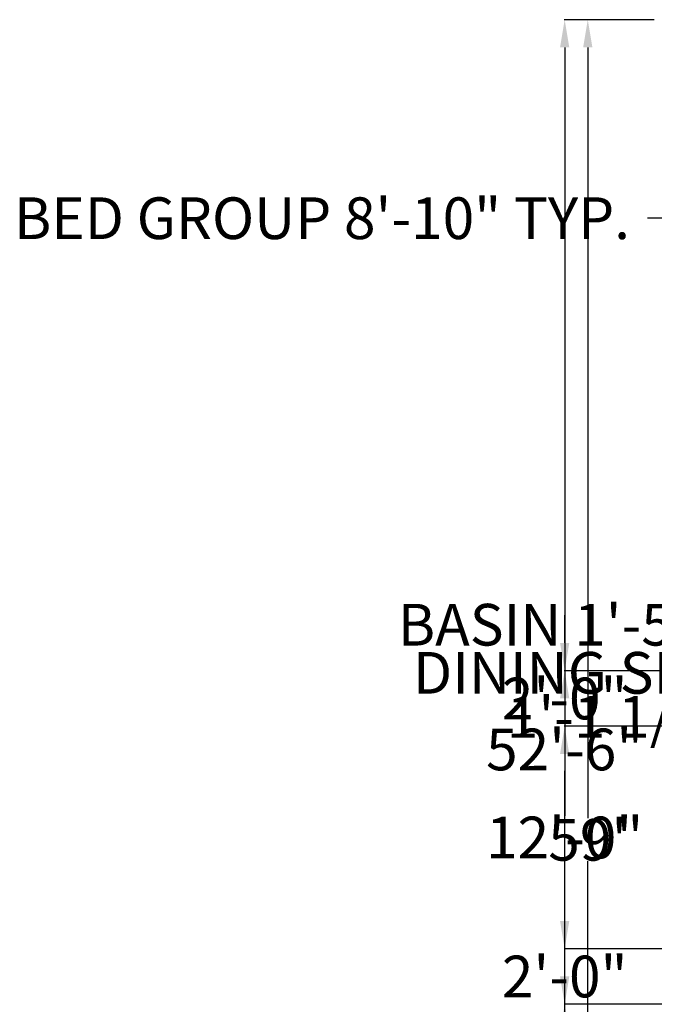
# Model space of a CAD drawing. Units: inches. Extents: x 2796 to 3603, y 978 to 1787.
# Tile 7 of 15: x 2796 to 3070, y 1312 to 1737. Entities that reach past the tile are written whole.
import ezdxf

# ---------------------------------------------------------------- set-up
doc = ezdxf.new("R2010")
doc.units = ezdxf.units.IN
doc.layers.add('A-ANNO-DIMS', color=7, linetype='Continuous', lineweight=18)
doc.styles.get("Standard").update_dxf_attribs({"font": 'arial.ttf'})
doc.dimstyles.get("Standard").update_dxf_attribs({"dimtxt": 18, "dimasz": 12, "dimexe": 0.18, "dimexo": 0.0625, "dimgap": 0.09, "dimtad": 0, "dimtih": 1, "dimtoh": 1, "dimdec": 0, "dimzin": 0, "dimdsep": 46, "dimlunit": 3, "dimtxsty": 'Standard', "dimcen": 0.09, "dimadec": 0, "dimazin": 0, "dimtfac": 1, "dimtdec": 0, "dimtofl": 0, "dimtmove": 0, "dimatfit": 3, "dimfxl": 1, "dimtolj": 1, "dimtzin": 0, "dimarcsym": 0})

# ---------------------------------------------------------------- blocks, each defined once
blk = doc.blocks.new('*D12')
at = {"layer": 'A-ANNO-DIMS', "color": 0, "lineweight": -2, "transparency": 16777216}
for p, q in [((3070.18, 1736.68), (3041.33, 1736.68)), ((3041.51, 1724.68), (3041.51, 1391.96)), ((3041.51, 1040.68), (3041.51, 1373.4)), ((3070.18, 1028.68), (3041.33, 1028.68))]:
    blk.add_line(p, q, dxfattribs=at)
at = {"layer": 'A-ANNO-DIMS', "color": 0, "transparency": 16777216}
for points in [[(3039.51, 1724.68), (3043.51, 1724.68), (3041.51, 1736.68)], [(3039.51, 1040.68), (3043.51, 1040.68), (3041.51, 1028.68)]]:
    blk.add_solid(points, dxfattribs=at)
at = {"layer": 'Defpoints', "color": 0, "transparency": 16777216}
for p in [(3041.51, 1736.68), (3070.25, 1736.68), (3070.25, 1028.68)]:
    blk.add_point(p, dxfattribs=at)
at = {"layer": 'A-ANNO-DIMS', "color": 0, "transparency": 16777216, "insert": (3041.51, 1382.68), "char_height": 18, "attachment_point": 5}
blk.add_mtext("\\A1;59'", dxfattribs=at)
blk = doc.blocks.new('*D22')
at = {"layer": 'A-ANNO-DIMS', "color": 0, "lineweight": -2, "transparency": 16777216}
for p, q in [((3160.28, 1475.52), (3148.28, 1475.52)), ((3172.28, 1473.07), (3172.28, 1475.7)), ((3189.07, 1473.07), (3189.07, 1475.7)), ((3201.07, 1475.52), (3213.07, 1475.52))]:
    blk.add_line(p, q, dxfattribs=at)
at = {"layer": 'A-ANNO-DIMS', "color": 0, "transparency": 16777216}
for points in [[(3160.28, 1477.52), (3160.28, 1473.52), (3172.28, 1475.52)], [(3201.07, 1477.52), (3201.07, 1473.52), (3189.07, 1475.52)]]:
    blk.add_solid(points, dxfattribs=at)
at = {"layer": 'Defpoints', "color": 0, "transparency": 16777216}
for p in [(3172.28, 1475.52), (3172.28, 1473), (3189.07, 1473)]:
    blk.add_point(p, dxfattribs=at)
at = {"layer": 'A-ANNO-DIMS', "color": 0, "transparency": 16777216, "insert": (3052.51, 1475.52), "char_height": 18, "attachment_point": 5}
blk.add_mtext('\\A1;BASIN 1\'-5" TYP.', dxfattribs=at)
blk = doc.blocks.new('*D23')
at = {"layer": 'A-ANNO-DIMS', "color": 0, "lineweight": -2, "transparency": 16777216}
for p, q in [((3169.76, 1485), (3169.76, 1497)), ((3172.22, 1473), (3169.58, 1473)), ((3172.22, 1459.7), (3169.58, 1459.7)), ((3169.76, 1447.7), (3169.76, 1435.7)), ((3169.76, 1435.7), (3157.76, 1435.7))]:
    blk.add_line(p, q, dxfattribs=at)
at = {"layer": 'A-ANNO-DIMS', "color": 0, "transparency": 16777216}
for points in [[(3167.76, 1485), (3171.76, 1485), (3169.76, 1473)], [(3167.76, 1447.7), (3171.76, 1447.7), (3169.76, 1459.7)]]:
    blk.add_solid(points, dxfattribs=at)
at = {"layer": 'Defpoints', "color": 0, "transparency": 16777216}
for p in [(3172.28, 1473), (3169.76, 1459.7), (3172.28, 1459.7)]:
    blk.add_point(p, dxfattribs=at)
at = {"layer": 'A-ANNO-DIMS', "color": 0, "transparency": 16777216, "insert": (3082.69, 1435.7), "char_height": 18, "attachment_point": 5}
blk.add_mtext('\\A1;1\'-1 1/2" TYP.', dxfattribs=at)
blk = doc.blocks.new('*D26')
at = {"layer": 'A-ANNO-DIMS', "color": 0, "lineweight": -2, "transparency": 16777216}
for p, q in [((3079.25, 1650.99), (3067.25, 1650.99)), ((3079.25, 1635.16), (3079.25, 1651.17)), ((3173.2, 1650.99), (3091.25, 1650.99)), ((3185.2, 1635.16), (3185.2, 1651.17))]:
    blk.add_line(p, q, dxfattribs=at)
at = {"layer": 'A-ANNO-DIMS', "color": 0, "transparency": 16777216}
for points in [[(3091.25, 1652.99), (3091.25, 1648.99), (3079.25, 1650.99)], [(3173.2, 1652.99), (3173.2, 1648.99), (3185.2, 1650.99)]]:
    blk.add_solid(points, dxfattribs=at)
at = {"layer": 'Defpoints', "color": 0, "transparency": 16777216}
for p in [(3079.25, 1650.99), (3079.25, 1635.1), (3185.2, 1635.1)]:
    blk.add_point(p, dxfattribs=at)
at = {"layer": 'A-ANNO-DIMS', "color": 0, "transparency": 16777216, "insert": (2926.76, 1650.99), "char_height": 18, "attachment_point": 5}
blk.add_mtext('\\A1;BED GROUP 8\'-10" TYP.', dxfattribs=at)
blk = doc.blocks.new('*D32')
at = {"layer": 'A-ANNO-DIMS', "color": 0, "lineweight": -2, "transparency": 16777216}
for p, q in [((3229.46, 1454.75), (3217.46, 1454.75)), ((3229.46, 1444.07), (3229.46, 1454.93)), ((3289.09, 1454.75), (3241.46, 1454.75)), ((3301.09, 1444.07), (3301.09, 1454.93))]:
    blk.add_line(p, q, dxfattribs=at)
at = {"layer": 'A-ANNO-DIMS', "color": 0, "transparency": 16777216}
for points in [[(3241.46, 1456.75), (3241.46, 1452.75), (3229.46, 1454.75)], [(3289.09, 1456.75), (3289.09, 1452.75), (3301.09, 1454.75)]]:
    blk.add_solid(points, dxfattribs=at)
at = {"layer": 'Defpoints', "color": 0, "transparency": 16777216}
for p in [(3229.46, 1454.75), (3229.46, 1444.01), (3301.09, 1444.01)]:
    blk.add_point(p, dxfattribs=at)
at = {"layer": 'A-ANNO-DIMS', "color": 0, "transparency": 16777216, "insert": (3090.48, 1454.75), "char_height": 18, "attachment_point": 5}
blk.add_mtext('\\A1;DINING SET 5\'-11 1/2"', dxfattribs=at)
blk = doc.blocks.new('*D41')
at = {"layer": 'A-ANNO-DIMS', "color": 0, "lineweight": -2, "transparency": 16777216}
for p, q in [((3079.18, 1455.68), (3031.37, 1455.68)), ((3031.55, 1443.68), (3031.55, 1392.96)), ((3031.55, 1323.68), (3031.55, 1374.4)), ((3079.18, 1311.68), (3031.37, 1311.68))]:
    blk.add_line(p, q, dxfattribs=at)
at = {"layer": 'A-ANNO-DIMS', "color": 0, "transparency": 16777216}
for points in [[(3029.55, 1443.68), (3033.55, 1443.68), (3031.55, 1455.68)], [(3029.55, 1323.68), (3033.55, 1323.68), (3031.55, 1311.68)]]:
    blk.add_solid(points, dxfattribs=at)
at = {"layer": 'Defpoints', "color": 0, "transparency": 16777216}
for p in [(3031.55, 1455.68), (3079.25, 1455.68), (3079.25, 1311.68)]:
    blk.add_point(p, dxfattribs=at)
at = {"layer": 'A-ANNO-DIMS', "color": 0, "transparency": 16777216, "insert": (3031.55, 1383.68), "char_height": 18, "attachment_point": 5}
blk.add_mtext('\\A1;12\'-0"', dxfattribs=at)
blk = doc.blocks.new('*D45')
at = {"layer": 'A-ANNO-DIMS', "color": 0, "lineweight": -2, "transparency": 16777216}
for p, q in [((3070.18, 1736.68), (3031.37, 1736.68)), ((3031.55, 1724.68), (3031.55, 1430.96)), ((3031.55, 1118.68), (3031.55, 1412.4)), ((3070.18, 1106.68), (3031.37, 1106.68))]:
    blk.add_line(p, q, dxfattribs=at)
at = {"layer": 'A-ANNO-DIMS', "color": 0, "transparency": 16777216}
for points in [[(3029.55, 1724.68), (3033.55, 1724.68), (3031.55, 1736.68)], [(3029.55, 1118.68), (3033.55, 1118.68), (3031.55, 1106.68)]]:
    blk.add_solid(points, dxfattribs=at)
at = {"layer": 'Defpoints', "color": 0, "transparency": 16777216}
for p in [(3031.55, 1736.68), (3070.25, 1736.68), (3070.25, 1106.68)]:
    blk.add_point(p, dxfattribs=at)
at = {"layer": 'A-ANNO-DIMS', "color": 0, "transparency": 16777216, "insert": (3031.55, 1421.68), "char_height": 18, "attachment_point": 5}
blk.add_mtext('\\A1;52\'-6"', dxfattribs=at)
blk = doc.blocks.new('*D52')
at = {"layer": 'A-ANNO-DIMS', "color": 0, "lineweight": -2, "transparency": 16777216}
for p, q in [((3031.545499, 1467.67534), (3031.545499, 1479.67534)), ((3127.182999, 1455.67534), (3031.365499, 1455.67534)), ((3127.182999, 1431.67534), (3031.365499, 1431.67534)), ((3031.545499, 1419.67534), (3031.545499, 1407.67534))]:
    blk.add_line(p, q, dxfattribs=at)
at = {"layer": 'A-ANNO-DIMS', "color": 0, "transparency": 16777216}
for points in [[(3029.545499, 1467.67534), (3033.545499, 1467.67534), (3031.545499, 1455.67534)], [(3029.545499, 1419.67534), (3033.545499, 1419.67534), (3031.545499, 1431.67534)]]:
    blk.add_solid(points, dxfattribs=at)
at = {"layer": 'Defpoints', "color": 0, "transparency": 16777216}
for p in [(3031.545499, 1455.67534), (3127.245499, 1455.67534), (3127.245499, 1431.67534)]:
    blk.add_point(p, dxfattribs=at)
at = {"layer": 'A-ANNO-DIMS', "color": 0, "transparency": 16777216, "insert": (3031.545499, 1443.67534), "char_height": 18, "attachment_point": 5}
blk.add_mtext('\\A1;2\'-0"', dxfattribs=at)
blk = doc.blocks.new('*D53')
at = {"layer": 'A-ANNO-DIMS', "color": 0, "lineweight": -2, "transparency": 16777216}
for p, q in [((3031.545499, 1347.67534), (3031.545499, 1359.67534)), ((3333.182999, 1335.67534), (3031.365499, 1335.67534)), ((3333.182999, 1311.67534), (3031.365499, 1311.67534)), ((3031.545499, 1299.67534), (3031.545499, 1287.67534))]:
    blk.add_line(p, q, dxfattribs=at)
at = {"layer": 'A-ANNO-DIMS', "color": 0, "transparency": 16777216}
for points in [[(3029.545499, 1347.67534), (3033.545499, 1347.67534), (3031.545499, 1335.67534)], [(3029.545499, 1299.67534), (3033.545499, 1299.67534), (3031.545499, 1311.67534)]]:
    blk.add_solid(points, dxfattribs=at)
at = {"layer": 'Defpoints', "color": 0, "transparency": 16777216}
for p in [(3031.545499, 1335.67534), (3333.245499, 1335.67534), (3333.245499, 1311.67534)]:
    blk.add_point(p, dxfattribs=at)
at = {"layer": 'A-ANNO-DIMS', "color": 0, "transparency": 16777216, "insert": (3031.545499, 1323.67534), "char_height": 18, "attachment_point": 5}
blk.add_mtext('\\A1;2\'-0"', dxfattribs=at)

msp = doc.modelspace()

# ---------------------------------------------------------------- dimensions: what is measured, and where the dimension line sits
at = {"layer": 'A-ANNO-DIMS'}
for base, p1, p2, override, picture, middle in [((3031.55, 1736.68), (3070.25, 1106.68), (3070.25, 1736.68), {"dimdec": 1, "dimlfac": 1, "dimrnd": 0, "dimzin": 1, "dimdsep": 46, "dimlunit": 4, "dimfrac": 2}, '*D45', (3031.55, 1421.68)), ((3041.51, 1736.68), (3070.25, 1028.68), (3070.25, 1736.68), {"dimclrd": 0, "dimclre": 0, "dimclrt": 0}, '*D12', (3041.51, 1382.68)), ((3031.55, 1455.68), (3127.25, 1431.68), (3127.25, 1455.68), {"dimdec": 1, "dimlfac": 1, "dimrnd": 0, "dimzin": 1, "dimdsep": 46, "dimlunit": 4, "dimfrac": 2}, '*D52', (3031.55, 1443.68)), ((3031.55, 1455.68), (3079.25, 1311.68), (3079.25, 1455.68), {"dimdec": 1, "dimlfac": 1, "dimrnd": 0, "dimzin": 1, "dimdsep": 46, "dimlunit": 4, "dimfrac": 2}, '*D41', (3031.55, 1383.68)), ((3031.55, 1335.68), (3333.25, 1311.68), (3333.25, 1335.68), {"dimdec": 1, "dimlfac": 1, "dimrnd": 0, "dimzin": 1, "dimdsep": 46, "dimlunit": 4, "dimfrac": 2}, '*D53', (3031.55, 1323.68))]:
    dim = msp.add_linear_dim(base=base, p1=p1, p2=p2, angle=90, dimstyle='Standard', override=override, dxfattribs=at)
    dim.commit()
    dim.dimension.update_dxf_attribs({"geometry": picture, "text_midpoint": middle})
for base, p1, p2, angle, text, picture, middle in [((3079.2455, 1650.9914), (3185.2001, 1635.0982), (3079.2455, 1635.0982), 180, 'BED GROUP <> TYP.', '*D26', (2926.7592, 1650.9914)), ((3172.28, 1475.52), (3189.07, 1473), (3172.28, 1473), 180, 'BASIN <> TYP.', '*D22', (3052.51, 1475.52)), ((3229.46, 1454.75), (3301.09, 1444.01), (3229.46, 1444.01), 180, 'DINING SET <>', '*D32', (3090.48, 1454.75)), ((3169.76, 1459.7), (3172.28, 1473), (3172.28, 1459.7), 270, '<> TYP.', '*D23', (3082.69, 1435.7))]:
    dim = msp.add_linear_dim(base=base, p1=p1, p2=p2, angle=angle, text=text, dimstyle='Standard', override={"dimdec": 1, "dimlfac": 1, "dimrnd": 0, "dimzin": 1, "dimdsep": 46, "dimlunit": 4, "dimfrac": 2}, dxfattribs=at)
    dim.commit()
    dim.dimension.update_dxf_attribs({"geometry": picture, "text_midpoint": middle})

doc.saveas('drawing.dxf')
